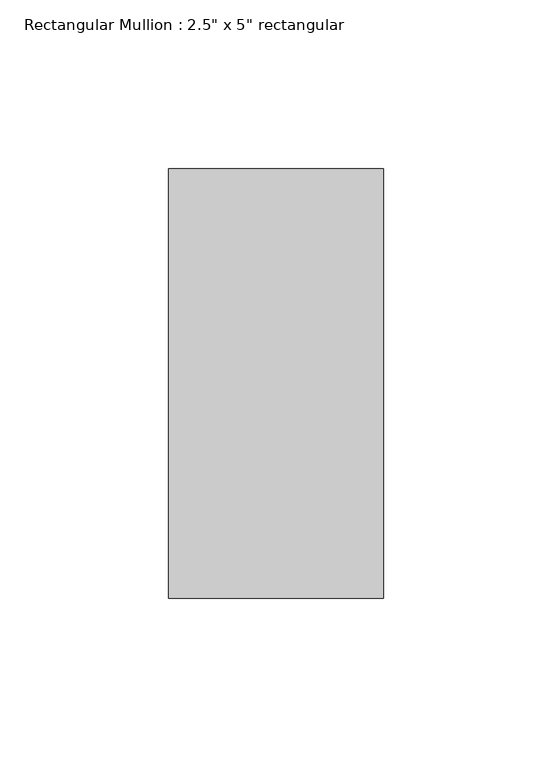
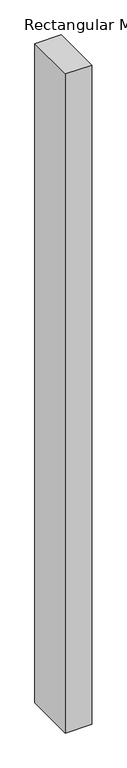
"""IFC4 building model written with IfcOpenShell, lengths in millimetres: member geometry."""

from ifc_helpers import new_model, si_unit, frame, origin, place, context, project, spatial, polyline, outline, extrude, source, transform, mapped, element, save


def member_530c9cc4(model_context):
    return source(origin(), model_context, "Body", "SweptSolid", [
        extrude(outline(polyline([(0.0, 63.5), (0.0, -63.5), (-63.5, -63.5), (-63.5, 63.5), (0.0, 63.5)])), frame((0.0, 0.0, -1682.0744644), z_axis=(0.0, 0.0, 1.0), x_axis=(1.0, 0.0, 0.0)), (0.0, 0.0, 1.0), 1682.0744644),
    ])


if __name__ == "__main__":
    model = new_model("IFC4")
    model_context = context("Model", 3, world=origin())
    ifc_project = project(units=[si_unit("LENGTHUNIT", "METRE", prefix="MILLI")], contexts=[model_context])
    site = spatial("IfcSite", under=ifc_project)
    building = spatial("IfcBuilding", under=site)
    placement = place(None, origin())
    member_shape = member_530c9cc4(model_context)
    element("IfcMember", 1, ObjectType="Rectangular Mullion : 2.5\" x 5\" rectangular", at=placement, inside=building, context=model_context, shape_type="MappedRepresentation", body=[
        mapped(member_shape, transform((0.0, 0.0, 0.0), x_axis=(1.0, 0.0, 0.0), y_axis=(0.0, 1.0, 0.0), z_axis=(0.0, 0.0, 1.0))),
    ])
    save(model, "model.ifc")

# Revit data of these elements
# Type "Rectangular Mullion : 2.5\" x 5\" rectangular"
#   built-in parameter 1007304 = 0.416667 (stored number, unit not read)
#   built-in parameter 1007301 = 0.104167 (stored number, unit not read)
#   built-in parameter 1007300 = 0.104167 (stored number, unit not read)
# Element 1 (IfcMember, "Rectangular Mullion : 2.5\" x 5\" rectangular")
#   Materials on its faces: "Aluminum"
# Materials
#   "Aluminum": class "Metal", colour RGB 247 247 247, transparency 0, Description = "Aluminum 6061", Cost = 0
